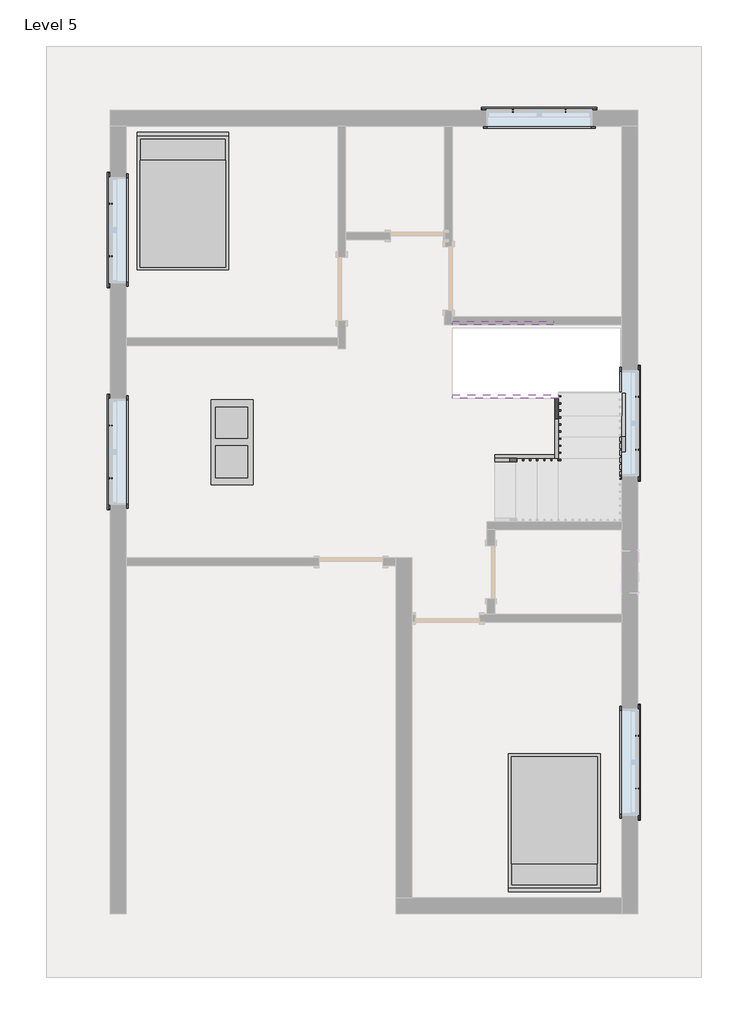
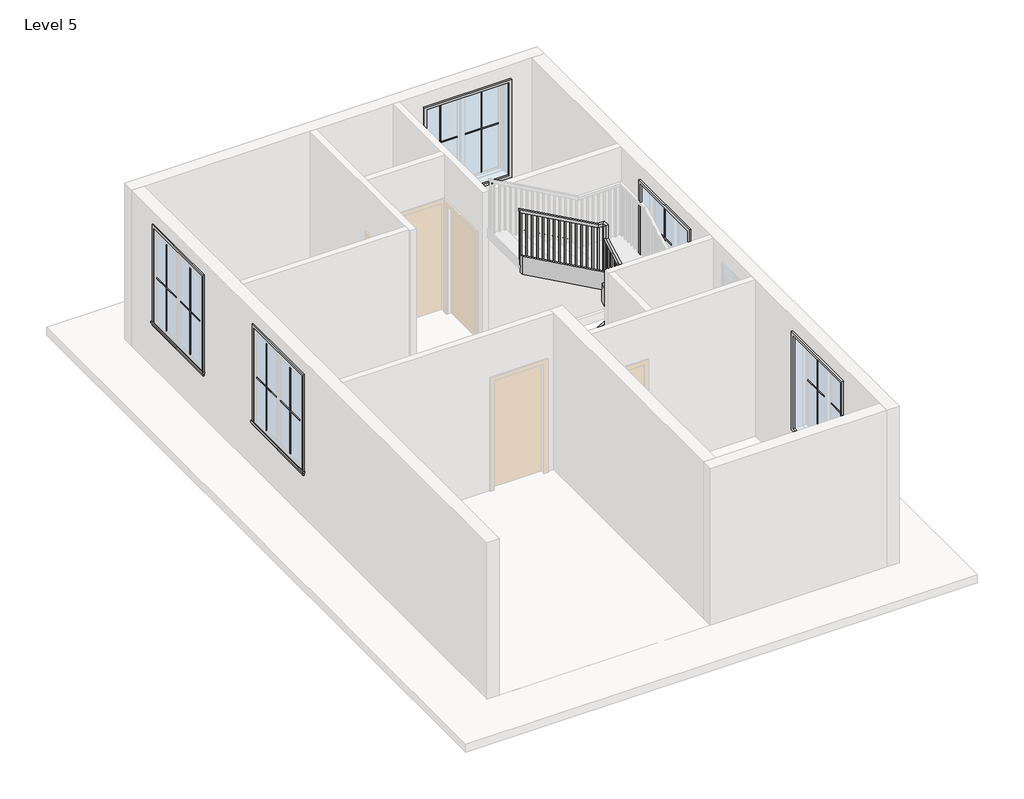
# One storey, part 2 of 2: 21 proxies, 6 members, 2 furniture elements, 1 railing.
"""IFC4 building model written with IfcOpenShell, lengths in millimetres."""

from ifc_helpers import new_model, si_unit, frame, origin, place, context, project, spatial, polyline, outline, extrude, faceted_brep, transform, mapped, element, save
from components import muntin_pattern_2x2_muntin_pattern_2x2_f6a80940, muntin_pattern_2x2_muntin_pattern_2x2_09b00a1c, trim_window_exterior_flat_with_sill_698ed857, trim_window_interior_flat_picture_frame_92551a5e, coffee_table_with_brass_mullions_11320_coffee_table_with_5962bef7, bed_17739_bed_17739_15c61121

model = new_model("IFC4")

# Units and contexts
model_context = context("Model", 3, world=origin())
ifc_project = project(units=[si_unit("LENGTHUNIT", "METRE", prefix="MILLI")], contexts=[model_context])

# Site, building, storey
site = spatial("IfcSite", under=ifc_project)
building = spatial("IfcBuilding", under=site)
storey = spatial("IfcBuildingStorey", under=building, Name="Level 5", Elevation=9601.2)

# Proxies
placement = place(None, origin())
muntin_pattern_2x2_muntin_pattern_2x2_shape = muntin_pattern_2x2_muntin_pattern_2x2_f6a80940(model_context)
element("IfcBuildingElementProxy", 1, Name="Muntin Pattern_2x2 : Muntin Pattern_2x2", ObjectType="Muntin Pattern_2x2 : Muntin Pattern_2x2", at=placement, inside=storey, context=model_context, shape_type="MappedRepresentation", body=[
    mapped(muntin_pattern_2x2_muntin_pattern_2x2_shape, transform((-4589.1575206, 441.8004493, 10585.45), x_axis=(0.0, 1.0, 0.0), y_axis=(-1.0, 0.0, 0.0), z_axis=(0.0, 0.0, 1.0))),
])
element("IfcBuildingElementProxy", 2, Name="Muntin Pattern_2x2 : Muntin Pattern_2x2", ObjectType="Muntin Pattern_2x2 : Muntin Pattern_2x2", at=placement, inside=storey, context=model_context, shape_type="MappedRepresentation", body=[
    mapped(muntin_pattern_2x2_muntin_pattern_2x2_shape, transform((-4589.1575206, 3632.6754493, 10585.45), x_axis=(0.0, 1.0, 0.0), y_axis=(-1.0, 0.0, 0.0), z_axis=(0.0, 0.0, 1.0))),
])
element("IfcBuildingElementProxy", 3, Name="Muntin Pattern_2x2 : Muntin Pattern_2x2", ObjectType="Muntin Pattern_2x2 : Muntin Pattern_2x2", at=placement, inside=storey, context=model_context, shape_type="MappedRepresentation", body=[
    mapped(muntin_pattern_2x2_muntin_pattern_2x2_shape, transform((1197.2799794, 5726.5879493, 10585.45), x_axis=(1.0, 0.0, 0.0), y_axis=(0.0, 1.0, 0.0), z_axis=(0.0, 0.0, 1.0))),
])
element("IfcBuildingElementProxy", 4, Name="Muntin Pattern_2x2 : Muntin Pattern_2x2", ObjectType="Muntin Pattern_2x2 : Muntin Pattern_2x2", at=placement, inside=storey, context=model_context, shape_type="MappedRepresentation", body=[
    mapped(muntin_pattern_2x2_muntin_pattern_2x2_shape, transform((2986.3924794, 1613.3754493, 10585.45), x_axis=(0.0, -1.0, 0.0), y_axis=(1.0, 0.0, 0.0), z_axis=(0.0, 0.0, 1.0))),
])
element("IfcBuildingElementProxy", 5, Name="Muntin Pattern_2x2 : Muntin Pattern_2x2", ObjectType="Muntin Pattern_2x2 : Muntin Pattern_2x2", at=placement, inside=storey, context=model_context, shape_type="MappedRepresentation", body=[
    mapped(muntin_pattern_2x2_muntin_pattern_2x2_shape, transform((2986.3924794, -3260.2495507, 10585.45), x_axis=(0.0, -1.0, 0.0), y_axis=(1.0, 0.0, 0.0), z_axis=(0.0, 0.0, 1.0))),
])
muntin_pattern_2x2_muntin_pattern_2x2_2_shape = muntin_pattern_2x2_muntin_pattern_2x2_09b00a1c(model_context)
element("IfcBuildingElementProxy", 6, Name="Muntin Pattern_2x2 : Muntin Pattern_2x2", ObjectType="Muntin Pattern_2x2 : Muntin Pattern_2x2", at=placement, inside=storey, context=model_context, shape_type="MappedRepresentation", body=[
    mapped(muntin_pattern_2x2_muntin_pattern_2x2_2_shape, transform((-4589.1575206, 1200.6254493, 10585.45), x_axis=(0.0, -1.0, 0.0), y_axis=(1.0, 0.0, 0.0), z_axis=(0.0, 0.0, 1.0))),
])
element("IfcBuildingElementProxy", 7, Name="Muntin Pattern_2x2 : Muntin Pattern_2x2", ObjectType="Muntin Pattern_2x2 : Muntin Pattern_2x2", at=placement, inside=storey, context=model_context, shape_type="MappedRepresentation", body=[
    mapped(muntin_pattern_2x2_muntin_pattern_2x2_2_shape, transform((-4589.1575206, 4391.5004493, 10585.45), x_axis=(0.0, -1.0, 0.0), y_axis=(1.0, 0.0, 0.0), z_axis=(0.0, 0.0, 1.0))),
])
element("IfcBuildingElementProxy", 8, Name="Muntin Pattern_2x2 : Muntin Pattern_2x2", ObjectType="Muntin Pattern_2x2 : Muntin Pattern_2x2", at=placement, inside=storey, context=model_context, shape_type="MappedRepresentation", body=[
    mapped(muntin_pattern_2x2_muntin_pattern_2x2_2_shape, transform((1956.1049794, 5726.5879493, 10585.45), x_axis=(-1.0, 0.0, 0.0), y_axis=(0.0, -1.0, 0.0), z_axis=(0.0, 0.0, 1.0))),
])
element("IfcBuildingElementProxy", 9, Name="Muntin Pattern_2x2 : Muntin Pattern_2x2", ObjectType="Muntin Pattern_2x2 : Muntin Pattern_2x2", at=placement, inside=storey, context=model_context, shape_type="MappedRepresentation", body=[
    mapped(muntin_pattern_2x2_muntin_pattern_2x2_2_shape, transform((2986.3924794, 854.5504493, 10585.45), x_axis=(0.0, 1.0, 0.0), y_axis=(-1.0, 0.0, 0.0), z_axis=(0.0, 0.0, 1.0))),
])
element("IfcBuildingElementProxy", 10, Name="Muntin Pattern_2x2 : Muntin Pattern_2x2", ObjectType="Muntin Pattern_2x2 : Muntin Pattern_2x2", at=placement, inside=storey, context=model_context, shape_type="MappedRepresentation", body=[
    mapped(muntin_pattern_2x2_muntin_pattern_2x2_2_shape, transform((2986.3924794, -4019.0745507, 10585.45), x_axis=(0.0, 1.0, 0.0), y_axis=(-1.0, 0.0, 0.0), z_axis=(0.0, 0.0, 1.0))),
])
trim_window_exterior_flat_with_sill_shape = trim_window_exterior_flat_with_sill_698ed857(model_context)
element("IfcBuildingElementProxy", 11, Name="Trim-Window-Exterior-Flat : with Sill", ObjectType="Trim-Window-Exterior-Flat : with Sill", at=placement, inside=storey, context=model_context, shape_type="MappedRepresentation", body=[
    mapped(trim_window_exterior_flat_with_sill_shape, transform((-4598.6825206, 821.2129493, 12344.4), x_axis=(0.0, -1.0, 0.0), y_axis=(0.0, 0.0, 1.0), z_axis=(-1.0, 0.0, 0.0))),
])
element("IfcBuildingElementProxy", 12, Name="Trim-Window-Exterior-Flat : with Sill", ObjectType="Trim-Window-Exterior-Flat : with Sill", at=placement, inside=storey, context=model_context, shape_type="MappedRepresentation", body=[
    mapped(trim_window_exterior_flat_with_sill_shape, transform((-4598.6825206, 4012.0879493, 12344.4), x_axis=(0.0, -1.0, 0.0), y_axis=(0.0, 0.0, 1.0), z_axis=(-1.0, 0.0, 0.0))),
])
element("IfcBuildingElementProxy", 13, Name="Trim-Window-Exterior-Flat : with Sill", ObjectType="Trim-Window-Exterior-Flat : with Sill", at=placement, inside=storey, context=model_context, shape_type="MappedRepresentation", body=[
    mapped(trim_window_exterior_flat_with_sill_shape, transform((1576.6924794, 5736.1129493, 12344.4), x_axis=(-1.0, 0.0, 0.0), y_axis=(0.0, 0.0, 1.0), z_axis=(0.0, 1.0, 0.0))),
])
element("IfcBuildingElementProxy", 14, Name="Trim-Window-Exterior-Flat : with Sill", ObjectType="Trim-Window-Exterior-Flat : with Sill", at=placement, inside=storey, context=model_context, shape_type="MappedRepresentation", body=[
    mapped(trim_window_exterior_flat_with_sill_shape, transform((2995.9174794, 1233.9629493, 12344.4), x_axis=(0.0, 1.0, 0.0), y_axis=(0.0, 0.0, 1.0), z_axis=(1.0, 0.0, 0.0))),
])
element("IfcBuildingElementProxy", 15, Name="Trim-Window-Exterior-Flat : with Sill", ObjectType="Trim-Window-Exterior-Flat : with Sill", at=placement, inside=storey, context=model_context, shape_type="MappedRepresentation", body=[
    mapped(trim_window_exterior_flat_with_sill_shape, transform((2995.9174794, -3639.6620507, 12344.4), x_axis=(0.0, 1.0, 0.0), y_axis=(0.0, 0.0, 1.0), z_axis=(1.0, 0.0, 0.0))),
])
trim_window_interior_flat_picture_frame_shape = trim_window_interior_flat_picture_frame_92551a5e(model_context)
element("IfcBuildingElementProxy", 16, Name="Trim-Window-Interior-Flat : Picture Frame", ObjectType="Trim-Window-Interior-Flat : Picture Frame", at=placement, inside=storey, context=model_context, shape_type="MappedRepresentation", body=[
    mapped(trim_window_interior_flat_picture_frame_shape, transform((-4370.0825206, 821.2129493, 12344.4), x_axis=(0.0, 1.0, 0.0), y_axis=(0.0, 0.0, 1.0), z_axis=(1.0, 0.0, 0.0))),
])
element("IfcBuildingElementProxy", 17, Name="Trim-Window-Interior-Flat : Picture Frame", ObjectType="Trim-Window-Interior-Flat : Picture Frame", at=placement, inside=storey, context=model_context, shape_type="MappedRepresentation", body=[
    mapped(trim_window_interior_flat_picture_frame_shape, transform((-4370.0825206, 4012.0879493, 12344.4), x_axis=(0.0, 1.0, 0.0), y_axis=(0.0, 0.0, 1.0), z_axis=(1.0, 0.0, 0.0))),
])
element("IfcBuildingElementProxy", 18, Name="Trim-Window-Interior-Flat : Picture Frame", ObjectType="Trim-Window-Interior-Flat : Picture Frame", at=placement, inside=storey, context=model_context, shape_type="MappedRepresentation", body=[
    mapped(trim_window_interior_flat_picture_frame_shape, transform((1576.6924794, 5507.5129493, 12344.4), x_axis=(1.0, 0.0, 0.0), y_axis=(0.0, 0.0, 1.0), z_axis=(0.0, -1.0, 0.0))),
])
element("IfcBuildingElementProxy", 19, Name="Trim-Window-Interior-Flat : Picture Frame", ObjectType="Trim-Window-Interior-Flat : Picture Frame", at=placement, inside=storey, context=model_context, shape_type="MappedRepresentation", body=[
    mapped(trim_window_interior_flat_picture_frame_shape, transform((2767.3174794, 1233.9629493, 12344.4), x_axis=(0.0, -1.0, 0.0), y_axis=(0.0, 0.0, 1.0), z_axis=(-1.0, 0.0, 0.0))),
])
element("IfcBuildingElementProxy", 20, Name="Trim-Window-Interior-Flat : Picture Frame", ObjectType="Trim-Window-Interior-Flat : Picture Frame", at=placement, inside=storey, context=model_context, shape_type="MappedRepresentation", body=[
    mapped(trim_window_interior_flat_picture_frame_shape, transform((2767.3174794, -3639.6620507, 12344.4), x_axis=(0.0, -1.0, 0.0), y_axis=(0.0, 0.0, 1.0), z_axis=(-1.0, 0.0, 0.0))),
])
coffee_table_with_brass_mullions_11320_coffee_table_with_shape = coffee_table_with_brass_mullions_11320_coffee_table_with_5962bef7(model_context)
element("IfcBuildingElementProxy", 21, Name="coffee_table_with_brass_mullions_11320 : coffee_table_with_brass_mullions_11320", ObjectType="coffee_table_with_brass_mullions_11320 : coffee_table_with_brass_mullions_11320", at=placement, inside=storey, context=model_context, shape_type="MappedRepresentation", body=[
    mapped(coffee_table_with_brass_mullions_11320_coffee_table_with_shape, transform((-2412.0418112, 1596.9678033, 9601.2), x_axis=(0.0, 1.0, 0.0), y_axis=(-1.0, 0.0, 0.0), z_axis=(0.0, 0.0, 1.0))),
])

# Furniture
bed_17739_bed_17739_shape = bed_17739_bed_17739_15c61121(model_context)
element("IfcFurniture", 22, ObjectType="Bed_17739 : Bed_17739", at=placement, inside=storey, context=model_context, shape_type="MappedRepresentation", body=[
    mapped(bed_17739_bed_17739_shape, transform((-3550.9325206, 4402.6129493, 9601.2), x_axis=(1.0, 0.0, 0.0), y_axis=(0.0, 1.0, 0.0), z_axis=(0.0, 0.0, 1.0))),
])
element("IfcFurniture", 23, ObjectType="Bed_17739 : Bed_17739", at=placement, inside=storey, context=model_context, shape_type="MappedRepresentation", body=[
    mapped(bed_17739_bed_17739_shape, transform((1795.7674794, -4487.3870507, 9601.2), x_axis=(-1.0, 0.0, 0.0), y_axis=(0.0, -1.0, 0.0), z_axis=(0.0, 0.0, 1.0))),
])

# Members
element("IfcMember", 24, ObjectType="Stringer - 2\" Width", at=placement, inside=storey, context=model_context, shape_type="SweptSolid", body=[
    extrude(outline(polyline([(9808.7983948, 938.5174794), (9601.2, 938.5174794), (9601.2, 1192.4619822), (9939.8974984, 1802.1174794), (10288.5761726, 1802.1174794), (9808.7983948, 938.5174794)])), frame((0.0, 732.3129493, 0.0), z_axis=(0.0, 1.0, 0.0), x_axis=(0.0, 0.0, 1.0)), (0.0, 0.0, 1.0), 50.8),
])
element("IfcMember", 25, ObjectType="Stringer - 2\" Width", at=placement, inside=storey, context=model_context, shape_type="SweptSolid", body=[
    extrude(outline(polyline([(732.3129493, 10137.453054), (732.3129493, 10486.1317281), (1595.9129493, 10965.9095059), (1595.9129493, 10617.2308318), (732.3129493, 10137.453054)])), frame((1802.1174794, 0.0, 0.0), z_axis=(1.0, 0.0, 0.0), x_axis=(0.0, 1.0, 0.0)), (0.0, 0.0, 1.0), 50.8),
])
element("IfcMember", 26, ObjectType="Stringer - 2\" Width", at=placement, inside=storey, context=model_context, shape_type="SweptSolid", body=[
    extrude(outline(polyline([(10814.7863873, 1852.9174794), (11163.4650614, 1852.9174794), (12010.1317281, 328.9174794), (11661.453054, 328.9174794), (10814.7863873, 1852.9174794)])), frame((0.0, 1595.9129493, 0.0), z_axis=(0.0, 1.0, 0.0), x_axis=(0.0, 0.0, 1.0)), (0.0, 0.0, 1.0), 50.8),
])
element("IfcMember", 27, ObjectType="Stringer - 2\" Width", at=placement, inside=storey, context=model_context, shape_type="SweptSolid", body=[
    extrude(outline(polyline([(9808.7983948, 938.5174794), (9601.2, 938.5174794), (9601.2, 1192.4619822), (9978.1317281, 1870.9390928), (9978.1317281, 1243.3174794), (9808.7983948, 938.5174794)])), frame((0.0, -232.8870507, 0.0), z_axis=(0.0, 1.0, 0.0), x_axis=(0.0, 0.0, 1.0)), (0.0, 0.0, 1.0), 50.8),
])
element("IfcMember", 28, ObjectType="Stringer - 2\" Width", at=placement, inside=storey, context=model_context, shape_type="SweptSolid", body=[
    extrude(outline(polyline([(714.2913359, 10476.1197207), (1037.1129493, 10655.4650614), (1664.7345627, 10655.4650614), (1341.9129493, 10476.1197207), (714.2913359, 10476.1197207)])), frame((2767.3174794, 0.0, 0.0), z_axis=(1.0, 0.0, 0.0), x_axis=(0.0, 1.0, 0.0)), (0.0, 0.0, 1.0), 50.8),
])
element("IfcMember", 29, ObjectType="Stringer - 2\" Width", at=placement, inside=storey, context=model_context, shape_type="SweptSolid", body=[
    extrude(outline(polyline([(11202.8419429, 1782.0390928), (12010.1317281, 328.9174794), (11661.453054, 328.9174794), (11202.8419429, 1154.4174794), (11202.8419429, 1782.0390928)])), frame((0.0, 2650.0129493, 0.0), z_axis=(0.0, 1.0, 0.0), x_axis=(0.0, 0.0, 1.0)), (0.0, 0.0, 1.0), 50.8),
])

# Railing
element("IfcRailing", 30, ObjectType="Handrail - Rectangular", at=placement, inside=storey, context=model_context, shape_type="SolidModel", body=[
    faceted_brep([(938.5174794, 732.3129493, 10684.9333333), (938.5174794, 732.3129493, 10626.820221), (938.5174794, 681.5129493, 10626.820221), (938.5174794, 681.5129493, 10684.9333333), (1776.7174794, 732.3129493, 11150.6), (1827.5174794, 732.3129493, 11120.7091099), (1827.5174794, 681.5129493, 11120.7091099), (1776.7174794, 681.5129493, 11150.6), (1776.7174794, 732.3129493, 11404.6), (1827.5174794, 732.3129493, 11353.8), (1827.5174794, 681.5129493, 11353.8), (1776.7174794, 681.5129493, 11404.6), (1852.9174794, 732.3129493, 11404.6), (1852.9174794, 732.3129493, 11353.8), (1903.7174794, 681.5129493, 11353.8), (1903.7174794, 681.5129493, 11404.6), (1852.9174794, 808.5129493, 11404.6), (1852.9174794, 821.6765516, 11353.8), (1903.7174794, 821.6765516, 11353.8), (1903.7174794, 808.5129493, 11404.6), (1852.9174794, 1570.5129493, 11827.9333333), (1852.9174794, 1621.3129493, 11798.0424432), (1903.7174794, 1621.3129493, 11798.0424432), (1903.7174794, 1570.5129493, 11827.9333333), (1852.9174794, 1570.5129493, 12081.9333333), (1852.9174794, 1621.3129493, 12031.1333333), (1903.7174794, 1621.3129493, 12031.1333333), (1903.7174794, 1570.5129493, 12081.9333333), (1852.9174794, 1646.7129493, 12081.9333333), (1852.9174794, 1646.7129493, 12031.1333333), (1903.7174794, 1697.5129493, 12031.1333333), (1903.7174794, 1697.5129493, 12081.9333333), (1776.7174794, 1646.7129493, 12081.9333333), (1763.5538772, 1646.7129493, 12031.1333333), (1763.5538772, 1697.5129493, 12031.1333333), (1776.7174794, 1697.5129493, 12081.9333333), (328.9174794, 1646.7129493, 12886.2666667), (328.9174794, 1697.5129493, 12886.2666667), (328.9174794, 1697.5129493, 12828.1535543), (328.9174794, 1646.7129493, 12828.1535543)], [[[0, 1, 2, 3]], [[1, 0, 4, 5]], [[2, 1, 5, 6]], [[3, 2, 6, 7]], [[0, 3, 7, 4]], [[5, 4, 8, 9]], [[6, 5, 9, 10]], [[7, 6, 10, 11]], [[4, 7, 11, 8]], [[9, 8, 12, 13]], [[10, 9, 13, 14]], [[11, 10, 14, 15]], [[8, 11, 15, 12]], [[13, 12, 16, 17]], [[14, 13, 17, 18]], [[15, 14, 18, 19]], [[12, 15, 19, 16]], [[17, 16, 20, 21]], [[18, 17, 21, 22]], [[19, 18, 22, 23]], [[16, 19, 23, 20]], [[21, 20, 24, 25]], [[22, 21, 25, 26]], [[23, 22, 26, 27]], [[20, 23, 27, 24]], [[25, 24, 28, 29]], [[26, 25, 29, 30]], [[27, 26, 30, 31]], [[24, 27, 31, 28]], [[29, 28, 32, 33]], [[30, 29, 33, 34]], [[31, 30, 34, 35]], [[28, 31, 35, 32]], [[36, 37, 38, 39]], [[33, 32, 36, 39]], [[34, 33, 39, 38]], [[35, 34, 38, 37]], [[32, 35, 37, 36]]]),
    extrude(outline(polyline([(12819.3341099, 344.7924794), (11802.5333333, 344.7924794), (11802.5333333, 363.8424794), (12808.7507765, 363.8424794), (12819.3341099, 344.7924794)])), frame((0.0, 1662.5879493, 0.0), z_axis=(0.0, 1.0, 0.0), x_axis=(0.0, 0.0, 1.0)), (0.0, 0.0, 1.0), 19.05),
    extrude(outline(polyline([(12762.8896654, 446.3924794), (11802.5333333, 446.3924794), (11802.5333333, 465.4424794), (12752.3063321, 465.4424794), (12762.8896654, 446.3924794)])), frame((0.0, 1662.5879493, 0.0), z_axis=(0.0, 1.0, 0.0), x_axis=(0.0, 0.0, 1.0)), (0.0, 0.0, 1.0), 19.05),
    extrude(outline(polyline([(12706.445221, 547.9924794), (11802.5333333, 547.9924794), (11802.5333333, 567.0424794), (12695.8618876, 567.0424794), (12706.445221, 547.9924794)])), frame((0.0, 1662.5879493, 0.0), z_axis=(0.0, 1.0, 0.0), x_axis=(0.0, 0.0, 1.0)), (0.0, 0.0, 1.0), 19.05),
    extrude(outline(polyline([(12650.0007765, 649.5924794), (11633.2, 649.5924794), (11633.2, 668.6424794), (12639.4174432, 668.6424794), (12650.0007765, 649.5924794)])), frame((0.0, 1662.5879493, 0.0), z_axis=(0.0, 1.0, 0.0), x_axis=(0.0, 0.0, 1.0)), (0.0, 0.0, 1.0), 19.05),
    extrude(outline(polyline([(12593.5563321, 751.1924794), (11633.2, 751.1924794), (11633.2, 770.2424794), (12582.9729988, 770.2424794), (12593.5563321, 751.1924794)])), frame((0.0, 1662.5879493, 0.0), z_axis=(0.0, 1.0, 0.0), x_axis=(0.0, 0.0, 1.0)), (0.0, 0.0, 1.0), 19.05),
    extrude(outline(polyline([(12537.1118876, 852.7924794), (11633.2, 852.7924794), (11633.2, 871.8424794), (12526.5285543, 871.8424794), (12537.1118876, 852.7924794)])), frame((0.0, 1662.5879493, 0.0), z_axis=(0.0, 1.0, 0.0), x_axis=(0.0, 0.0, 1.0)), (0.0, 0.0, 1.0), 19.05),
    extrude(outline(polyline([(12480.6674432, 954.3924794), (11463.8666667, 954.3924794), (11463.8666667, 973.4424794), (12470.0841099, 973.4424794), (12480.6674432, 954.3924794)])), frame((0.0, 1662.5879493, 0.0), z_axis=(0.0, 1.0, 0.0), x_axis=(0.0, 0.0, 1.0)), (0.0, 0.0, 1.0), 19.05),
    extrude(outline(polyline([(12424.2229988, 1055.9924794), (11463.8666667, 1055.9924794), (11463.8666667, 1075.0424794), (12413.6396654, 1075.0424794), (12424.2229988, 1055.9924794)])), frame((0.0, 1662.5879493, 0.0), z_axis=(0.0, 1.0, 0.0), x_axis=(0.0, 0.0, 1.0)), (0.0, 0.0, 1.0), 19.05),
    extrude(outline(polyline([(12367.7785543, 1157.5924794), (11463.8666667, 1157.5924794), (11463.8666667, 1176.6424794), (12357.195221, 1176.6424794), (12367.7785543, 1157.5924794)])), frame((0.0, 1662.5879493, 0.0), z_axis=(0.0, 1.0, 0.0), x_axis=(0.0, 0.0, 1.0)), (0.0, 0.0, 1.0), 19.05),
    extrude(outline(polyline([(12311.3341099, 1259.1924794), (11294.5333333, 1259.1924794), (11294.5333333, 1278.2424794), (12300.7507765, 1278.2424794), (12311.3341099, 1259.1924794)])), frame((0.0, 1662.5879493, 0.0), z_axis=(0.0, 1.0, 0.0), x_axis=(0.0, 0.0, 1.0)), (0.0, 0.0, 1.0), 19.05),
    extrude(outline(polyline([(12254.8896654, 1360.7924794), (11294.5333333, 1360.7924794), (11294.5333333, 1379.8424794), (12244.3063321, 1379.8424794), (12254.8896654, 1360.7924794)])), frame((0.0, 1662.5879493, 0.0), z_axis=(0.0, 1.0, 0.0), x_axis=(0.0, 0.0, 1.0)), (0.0, 0.0, 1.0), 19.05),
    extrude(outline(polyline([(12198.445221, 1462.3924794), (11294.5333333, 1462.3924794), (11294.5333333, 1481.4424794), (12187.8618876, 1481.4424794), (12198.445221, 1462.3924794)])), frame((0.0, 1662.5879493, 0.0), z_axis=(0.0, 1.0, 0.0), x_axis=(0.0, 0.0, 1.0)), (0.0, 0.0, 1.0), 19.05),
    extrude(outline(polyline([(12142.0007765, 1563.9924794), (11125.2, 1563.9924794), (11125.2, 1583.0424794), (12131.4174432, 1583.0424794), (12142.0007765, 1563.9924794)])), frame((0.0, 1662.5879493, 0.0), z_axis=(0.0, 1.0, 0.0), x_axis=(0.0, 0.0, 1.0)), (0.0, 0.0, 1.0), 19.05),
    extrude(outline(polyline([(12085.5563321, 1665.5924794), (11125.2, 1665.5924794), (11125.2, 1684.6424794), (12074.9729988, 1684.6424794), (12085.5563321, 1665.5924794)])), frame((0.0, 1662.5879493, 0.0), z_axis=(0.0, 1.0, 0.0), x_axis=(0.0, 0.0, 1.0)), (0.0, 0.0, 1.0), 19.05),
    extrude(outline(polyline([(12029.1118876, 1767.1924794), (11125.2, 1767.1924794), (11125.2, 1786.2424794), (12018.5285543, 1786.2424794), (12029.1118876, 1767.1924794)])), frame((0.0, 1662.5879493, 0.0), z_axis=(0.0, 1.0, 0.0), x_axis=(0.0, 0.0, 1.0)), (0.0, 0.0, 1.0), 19.05),
    extrude(outline(polyline([(1868.7924794, 1611.7879493), (1868.7924794, 1630.8379493), (1887.8424794, 1630.8379493), (1887.8424794, 1611.7879493), (1868.7924794, 1611.7879493)])), frame((0.0, 0.0, 10786.5333333), z_axis=(0.0, 0.0, 1.0), x_axis=(1.0, 0.0, 0.0)), (0.0, 0.0, 1.0), 1244.6),
    extrude(outline(polyline([(1529.2379493, 11746.8896654), (1529.2379493, 10786.5333333), (1510.1879493, 10786.5333333), (1510.1879493, 11736.3063321), (1529.2379493, 11746.8896654)])), frame((1868.7924794, 0.0, 0.0), z_axis=(1.0, 0.0, 0.0), x_axis=(0.0, 1.0, 0.0)), (0.0, 0.0, 1.0), 19.05),
    extrude(outline(polyline([(1427.6379493, 11690.445221), (1427.6379493, 10786.5333333), (1408.5879493, 10786.5333333), (1408.5879493, 11679.8618876), (1427.6379493, 11690.445221)])), frame((1868.7924794, 0.0, 0.0), z_axis=(1.0, 0.0, 0.0), x_axis=(0.0, 1.0, 0.0)), (0.0, 0.0, 1.0), 19.05),
    extrude(outline(polyline([(1326.0379493, 11634.0007765), (1326.0379493, 10617.2), (1306.9879493, 10617.2), (1306.9879493, 11623.4174432), (1326.0379493, 11634.0007765)])), frame((1868.7924794, 0.0, 0.0), z_axis=(1.0, 0.0, 0.0), x_axis=(0.0, 1.0, 0.0)), (0.0, 0.0, 1.0), 19.05),
    extrude(outline(polyline([(1224.4379493, 11577.5563321), (1224.4379493, 10617.2), (1205.3879493, 10617.2), (1205.3879493, 11566.9729988), (1224.4379493, 11577.5563321)])), frame((1868.7924794, 0.0, 0.0), z_axis=(1.0, 0.0, 0.0), x_axis=(0.0, 1.0, 0.0)), (0.0, 0.0, 1.0), 19.05),
    extrude(outline(polyline([(1122.8379493, 11521.1118876), (1122.8379493, 10617.2), (1103.7879493, 10617.2), (1103.7879493, 11510.5285543), (1122.8379493, 11521.1118876)])), frame((1868.7924794, 0.0, 0.0), z_axis=(1.0, 0.0, 0.0), x_axis=(0.0, 1.0, 0.0)), (0.0, 0.0, 1.0), 19.05),
    extrude(outline(polyline([(1021.2379493, 11464.6674432), (1021.2379493, 10447.8666667), (1002.1879493, 10447.8666667), (1002.1879493, 11454.0841099), (1021.2379493, 11464.6674432)])), frame((1868.7924794, 0.0, 0.0), z_axis=(1.0, 0.0, 0.0), x_axis=(0.0, 1.0, 0.0)), (0.0, 0.0, 1.0), 19.05),
    extrude(outline(polyline([(919.6379493, 11408.2229988), (919.6379493, 10447.8666667), (900.5879493, 10447.8666667), (900.5879493, 11397.6396654), (919.6379493, 11408.2229988)])), frame((1868.7924794, 0.0, 0.0), z_axis=(1.0, 0.0, 0.0), x_axis=(0.0, 1.0, 0.0)), (0.0, 0.0, 1.0), 19.05),
    extrude(outline(polyline([(818.0379493, 11351.7785543), (818.0379493, 10447.8666667), (798.9879493, 10447.8666667), (798.9879493, 11341.195221), (818.0379493, 11351.7785543)])), frame((1868.7924794, 0.0, 0.0), z_axis=(1.0, 0.0, 0.0), x_axis=(0.0, 1.0, 0.0)), (0.0, 0.0, 1.0), 19.05),
    extrude(outline(polyline([(1843.3924794, 716.4379493), (1862.4424794, 716.4379493), (1862.4424794, 697.3879493), (1843.3924794, 697.3879493), (1843.3924794, 716.4379493)])), frame((0.0, 0.0, 10278.5333333), z_axis=(0.0, 0.0, 1.0), x_axis=(1.0, 0.0, 0.0)), (0.0, 0.0, 1.0), 1075.2666667),
    extrude(outline(polyline([(11073.0841099, 1741.7924794), (10109.2, 1741.7924794), (10109.2, 1760.8424794), (11083.6674432, 1760.8424794), (11073.0841099, 1741.7924794)])), frame((0.0, 697.3879493, 0.0), z_axis=(0.0, 1.0, 0.0), x_axis=(0.0, 0.0, 1.0)), (0.0, 0.0, 1.0), 19.05),
    extrude(outline(polyline([(11016.6396654, 1640.1924794), (10109.2, 1640.1924794), (10109.2, 1659.2424794), (11027.2229988, 1659.2424794), (11016.6396654, 1640.1924794)])), frame((0.0, 697.3879493, 0.0), z_axis=(0.0, 1.0, 0.0), x_axis=(0.0, 0.0, 1.0)), (0.0, 0.0, 1.0), 19.05),
    extrude(outline(polyline([(10960.195221, 1538.5924794), (10109.2, 1538.5924794), (10109.2, 1557.6424794), (10970.7785543, 1557.6424794), (10960.195221, 1538.5924794)])), frame((0.0, 697.3879493, 0.0), z_axis=(0.0, 1.0, 0.0), x_axis=(0.0, 0.0, 1.0)), (0.0, 0.0, 1.0), 19.05),
    extrude(outline(polyline([(10903.7507765, 1436.9924794), (9939.8666667, 1436.9924794), (9939.8666667, 1456.0424794), (10914.3341099, 1456.0424794), (10903.7507765, 1436.9924794)])), frame((0.0, 697.3879493, 0.0), z_axis=(0.0, 1.0, 0.0), x_axis=(0.0, 0.0, 1.0)), (0.0, 0.0, 1.0), 19.05),
    extrude(outline(polyline([(10847.3063321, 1335.3924794), (9939.8666667, 1335.3924794), (9939.8666667, 1354.4424794), (10857.8896654, 1354.4424794), (10847.3063321, 1335.3924794)])), frame((0.0, 697.3879493, 0.0), z_axis=(0.0, 1.0, 0.0), x_axis=(0.0, 0.0, 1.0)), (0.0, 0.0, 1.0), 19.05),
    extrude(outline(polyline([(10790.8618876, 1233.7924794), (9939.8666667, 1233.7924794), (9939.8666667, 1252.8424794), (10801.445221, 1252.8424794), (10790.8618876, 1233.7924794)])), frame((0.0, 697.3879493, 0.0), z_axis=(0.0, 1.0, 0.0), x_axis=(0.0, 0.0, 1.0)), (0.0, 0.0, 1.0), 19.05),
    extrude(outline(polyline([(10734.4174432, 1132.1924794), (9770.5333333, 1132.1924794), (9770.5333333, 1151.2424794), (10745.0007765, 1151.2424794), (10734.4174432, 1132.1924794)])), frame((0.0, 697.3879493, 0.0), z_axis=(0.0, 1.0, 0.0), x_axis=(0.0, 0.0, 1.0)), (0.0, 0.0, 1.0), 19.05),
    extrude(outline(polyline([(10677.9729988, 1030.5924794), (9770.5333333, 1030.5924794), (9770.5333333, 1049.6424794), (10688.5563321, 1049.6424794), (10677.9729988, 1030.5924794)])), frame((0.0, 697.3879493, 0.0), z_axis=(0.0, 1.0, 0.0), x_axis=(0.0, 0.0, 1.0)), (0.0, 0.0, 1.0), 19.05),
    extrude(outline(polyline([(1868.7924794, 1662.5879493), (1868.7924794, 1681.6379493), (1887.8424794, 1681.6379493), (1887.8424794, 1662.5879493), (1868.7924794, 1662.5879493)])), frame((0.0, 0.0, 10955.8666667), z_axis=(0.0, 0.0, 1.0), x_axis=(1.0, 0.0, 0.0)), (0.0, 0.0, 1.0), 1075.2666667),
    extrude(outline(polyline([(1868.7924794, 716.4379493), (1887.8424794, 716.4379493), (1887.8424794, 697.3879493), (1868.7924794, 697.3879493), (1868.7924794, 716.4379493)])), frame((0.0, 0.0, 10278.5333333), z_axis=(0.0, 0.0, 1.0), x_axis=(1.0, 0.0, 0.0)), (0.0, 0.0, 1.0), 1075.2666667),
    extrude(outline(polyline([(12828.1535543, 328.9174794), (11802.5333333, 328.9174794), (11802.5333333, 347.9674794), (12817.570221, 347.9674794), (12828.1535543, 328.9174794)])), frame((0.0, 1662.5879493, 0.0), z_axis=(0.0, 1.0, 0.0), x_axis=(0.0, 0.0, 1.0)), (0.0, 0.0, 1.0), 19.05),
    extrude(outline(polyline([(10626.820221, 938.5174794), (9770.5333333, 938.5174794), (9770.5333333, 957.5674794), (10637.4035543, 957.5674794), (10626.820221, 938.5174794)])), frame((0.0, 697.3879493, 0.0), z_axis=(0.0, 1.0, 0.0), x_axis=(0.0, 0.0, 1.0)), (0.0, 0.0, 1.0), 19.05),
])

save(model, "model.ifc")

# Revit data of these elements
# Type "Muntin Pattern_2x2 : Muntin Pattern_2x2"
#   Width [instance default] = 4' - 0"
#   Thickness = 0' - 0 1/2"
#   Height [instance default] = 4' - 0"
#   Distance = 0' - 0 3/4"
#   Interior Material [instance default] = none
#   Exterior Material [instance default] = none
#   Default Elevation = 0
# Type "Trim-Window-Exterior-Flat : with Sill"
#   Trim Width = 0' - 2 1/4"
#   Trim Thickness_Picture Frame = 0' - 1 1/4"
#   Trim Thickness_with Sill = 0' - 0 3/4"
#   Sill Thickness = 0' - 1 1/4"
#   Opening Width [instance default] = 2' - 0"
#   Opening Height [instance default] = 3' - 0"
#   Default Elevation = 4' - 0"
#   Sill = yes
#   Picture Frame = no
#   Trim Material [instance default] = none
# Type "Trim-Window-Interior-Flat : Picture Frame"
#   Trim Thickness_Picture Frame = 0' - 1 1/4"
#   Trim Width = 0' - 2 1/4"
#   Trim Thickness_with Sill = 0' - 0 3/4"
#   Sill Thickness = 0' - 1 1/4"
#   Opening Width [instance default] = 2' - 0"
#   Opening Height [instance default] = 3' - 0"
#   Default Elevation = 4' - 0"
#   Sill = no
#   Picture Frame = yes
#   Trim Material [instance default] = none
# Type "coffee_table_with_brass_mullions_11320 : coffee_table_with_brass_mullions_11320"
#   Default Elevation = 0
# Type "Bed_17739 : Bed_17739"
#   Default Elevation = 0
# Type "Handrail - Rectangular"
#   Assembly Code = "C2010400"
#   built-in parameter 1008612 = 0.0416667 (stored number, unit not read)
#   built-in parameter 1008611 = 0.0416667 (stored number, unit not read)
#   built-in parameter 1008609 = 0.333333 (stored number, unit not read)
#   built-in parameter 1008604 = 0.166667 (stored number, unit not read)
#   built-in parameter 1008603 = 0.166667 (stored number, unit not read)
#   Railing Height = 3' - 0"
#   built-in parameter 1008630 = 2
#   built-in parameter 1008610 = 2
#   built-in parameter 1008618 = Baluster - Square : 3/4"
# Elements 1, 2, 3, 4, 5, 6, 7, 8, 9, 10 (IfcBuildingElementProxy, "Muntin Pattern_2x2 : Muntin Pattern_2x2")
#   Width = 2' - 0 5/8"
#   Height = 5' - 6 1/2"
#   Interior Material = Wood - Stained
#   Exterior Material = Clad - White
#   Phase Created = New Construction
#   Materials on its faces: "Clad - White", "Wood - Stained"
# Elements 11, 12, 13, 14, 15 (IfcBuildingElementProxy, "Trim-Window-Exterior-Flat : with Sill")
#   Opening Width = 5' - 0"
#   Opening Height = 6' - 0"
#   Trim Material = Clad - White
#   Phase Created = New Construction
#   Materials on its faces: "Clad - White"
# Elements 16, 17, 18, 19, 20 (IfcBuildingElementProxy, "Trim-Window-Interior-Flat : Picture Frame")
#   Opening Width = 5' - 0"
#   Opening Height = 6' - 0"
#   Trim Material = Wood - Stained
#   Phase Created = New Construction
#   Materials on its faces: "Wood - Stained"
# Element 21 (IfcBuildingElementProxy, "coffee_table_with_brass_mullions_11320 : coffee_table_with_brass_mullions_11320")
#   Phase Created = New Construction
#   Materials on its faces: "Default Wall", "TABLE", "Glass", "Default"
# Elements 22, 23 (IfcFurniture, "Bed_17739 : Bed_17739")
#   Phase Created = New Construction
#   Materials on its faces: "legs", "sheets", "bed frame", "Blanket"
# Elements 24, 25, 26, 27, 28, 29 (IfcMember, "Stringer - 2\" Width")
#   Phase Created = New Construction
# Element 30 (IfcRailing, "Handrail - Rectangular")
#   Phase Created = New Construction
# Materials
#   "Clad - White": class "Wood", colour RGB 242 242 238, transparency 0, Cost = 0
#   "Wood - Stained": class "Wood", colour RGB 224 178 126, transparency 0, Cost = 0
#   "Default Wall": colour RGB 128 128 128, transparency 0, Cost = 0
#   "TABLE": class "Generic", colour RGB 120 120 120, transparency 0, Cost = 0
#   "Glass": class "Glass", colour RGB 0 128 192, transparency 0.75, Description = "Soda Lime Glass", Cost = 0
#   "Default": colour RGB 127 127 127, transparency 0, Cost = 0
#   "legs": colour RGB 90 73 37, transparency 0, Cost = 0
#   "sheets": colour RGB 200 195 176, transparency 0, Cost = 0
#   "bed frame": colour RGB 90 73 37, transparency 0, Cost = 0
#   "Blanket": class "System", colour RGB 59 0 1, transparency 0, Cost = 0
